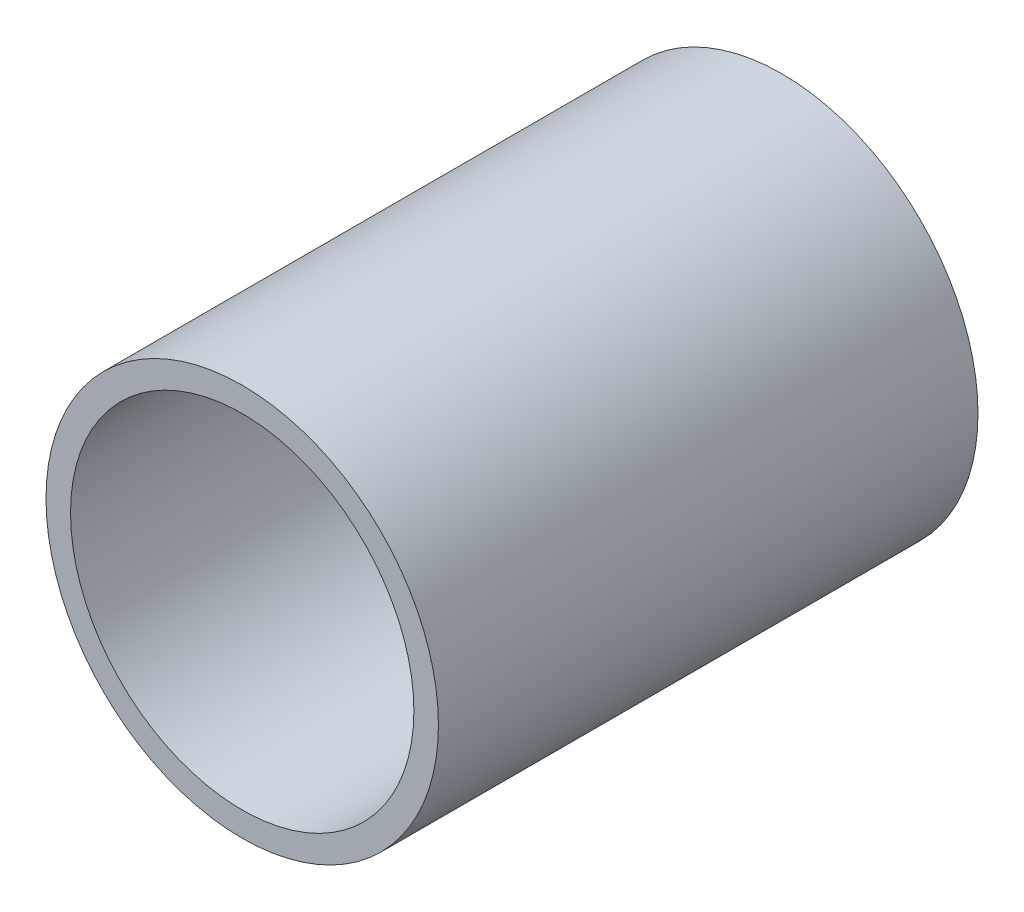
SolidWorks part; units mm, degrees
material "Plain Carbon Steel"
ref_plane "Front Plane" through (0, 0, 0) normal (0, 0, 1) x (1, 0, 0)
ref_plane "Top Plane" through (0, 0, 0) normal (0, 1, 0) x (1, 0, 0)
ref_plane "Right Plane" through (0, 0, 0) normal (1, 0, 0) x (0, 0, -1)
sketch "Sleeve Profile Ø80xØ70" plane through (0, 0, 0) normal (0, 0, 1) x (1, 0, 0)
  circle A0 centre (0, 0) radius 40
  circle A1 centre (0, 0) radius 35
  dimension "D1" = 80
  dimension "D2" = 70
extrude "Sleeve Body L110" add sketch "Sleeve Profile Ø80xØ70" along normal blind 110
